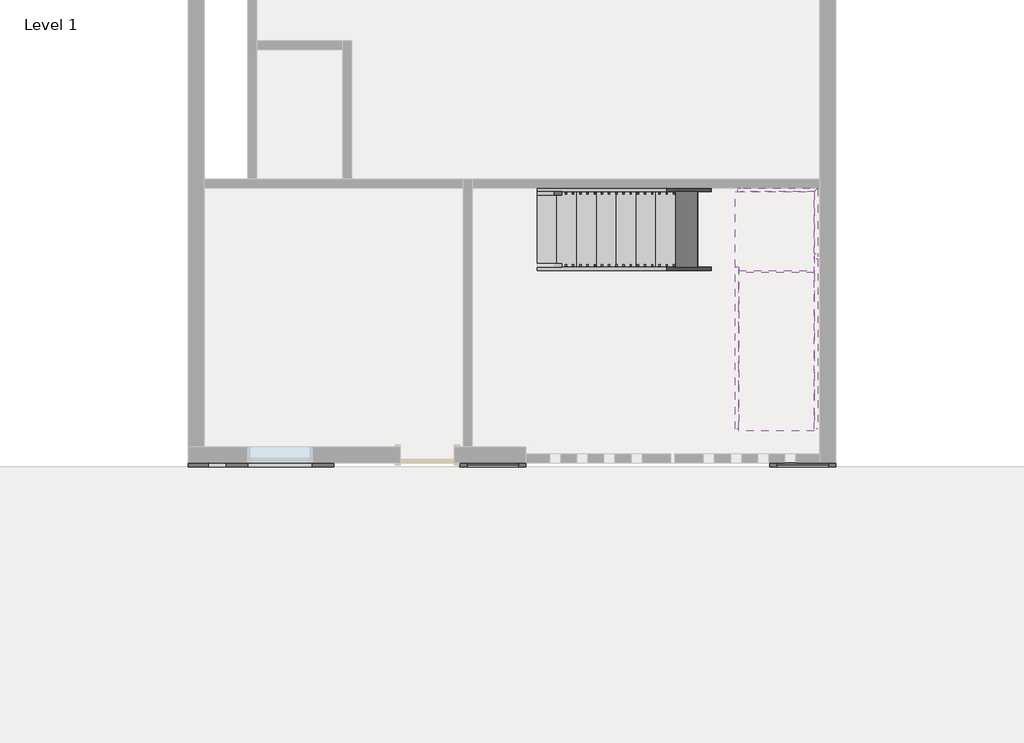
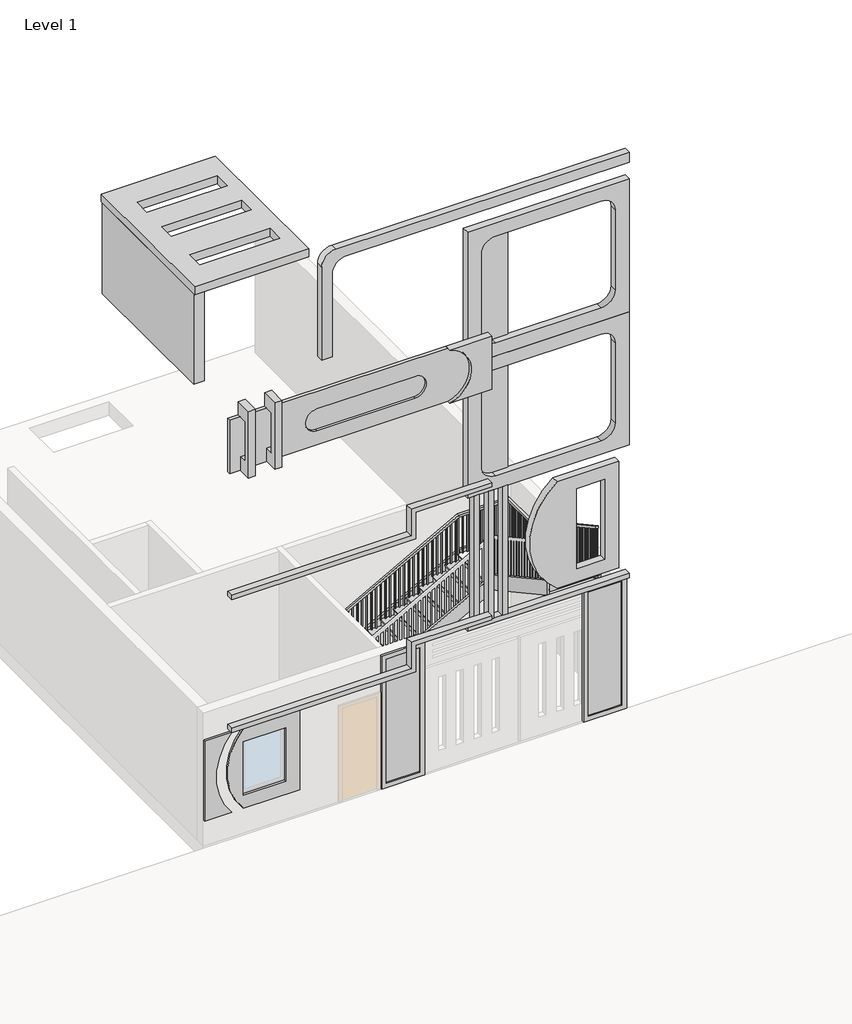
# One storey, part 2 of 2: 6 members, 2 stair flights, 1 proxy, 1 railing, 1 slab.
"""IFC4 building model written with IfcOpenShell, lengths in millimetres."""

from ifc_helpers import new_model, si_unit, frame, origin, place, context, project, spatial, polyline, outline, extrude, faceted_brep, transform, mapped, element, save
from components import generic_models_1_generic_models_1_57c6c2c0, non_monolithic_landing_2a78468c, stair_flight_cc90426c, stair_flight_f2f674f0

model = new_model("IFC4")

# Units and contexts
model_context = context("Model", 3, world=origin())
ifc_project = project(units=[si_unit("LENGTHUNIT", "METRE", prefix="MILLI")], contexts=[model_context])

# Site, building, storey
site = spatial("IfcSite", under=ifc_project)
building = spatial("IfcBuilding", under=site)
storey = spatial("IfcBuildingStorey", under=building, Name="Level 1", Elevation=0.0)

# Proxy
placement = place(None, origin())
generic_models_1_generic_models_1_shape = generic_models_1_generic_models_1_57c6c2c0(model_context)
element("IfcBuildingElementProxy", 1, Name="Generic Models 1 : Generic Models 1", ObjectType="Generic Models 1 : Generic Models 1", at=placement, inside=storey, context=model_context, shape_type="MappedRepresentation", body=[
    mapped(generic_models_1_generic_models_1_shape, transform((0.0, 0.0, 0.0), x_axis=(1.0, 0.0, 0.0), y_axis=(0.0, 1.0, 0.0), z_axis=(0.0, 0.0, 1.0))),
])

# Members
element("IfcMember", 2, ObjectType="Stringer - 2\" Width", at=placement, inside=storey, context=model_context, shape_type="SweptSolid", body=[
    extrude(outline(polyline([(206.7436667, -459.26646), (0.0, -459.26646), (0.0, -201.7743401), (1447.8, 2452.5256599), (1752.6, 2374.8034844), (206.7436667, -459.26646)])), frame((0.0, -782.3834702, 0.0), z_axis=(0.0, 1.0, 0.0), x_axis=(0.0, 0.0, 1.0)), (0.0, 0.0, 1.0), 50.8),
])
element("IfcMember", 3, ObjectType="Stringer - 2\" Width", at=placement, inside=storey, context=model_context, shape_type="SweptSolid", body=[
    extrude(outline(polyline([(206.7436667, -459.26646), (0.0, -459.26646), (0.0, -201.7743401), (1383.5497528, 2334.73354), (1730.7436667, 2334.73354), (206.7436667, -459.26646)])), frame((0.0, -1899.9834702, 0.0), z_axis=(0.0, 1.0, 0.0), x_axis=(0.0, 0.0, 1.0)), (0.0, 0.0, 1.0), 50.8),
])
element("IfcMember", 4, ObjectType="Stringer - 2\" Width", at=placement, inside=storey, context=model_context, shape_type="SweptSolid", body=[
    extrude(outline(polyline([(-1660.6534146, 1752.6), (-1738.3755901, 1447.8), (-4135.1834702, 2755.1497528), (-4135.1834702, 3102.3436667), (-1660.6534146, 1752.6)])), frame((3452.33354, 0.0, 0.0), z_axis=(1.0, 0.0, 0.0), x_axis=(0.0, 1.0, 0.0)), (0.0, 0.0, 1.0), 50.8),
])
element("IfcMember", 5, ObjectType="Stringer - 2\" Width", at=placement, inside=storey, context=model_context, shape_type="SweptSolid", body=[
    extrude(outline(polyline([(-1849.1834702, 1855.4345758), (-1849.1834702, 1508.2406619), (-4135.1834702, 2755.1497528), (-4135.1834702, 3102.3436667), (-1849.1834702, 1855.4345758)])), frame((2334.73354, 0.0, 0.0), z_axis=(1.0, 0.0, 0.0), x_axis=(0.0, 1.0, 0.0)), (0.0, 0.0, 1.0), 50.8),
])
element("IfcMember", 6, ObjectType="Stringer - 2\" Width", at=placement, inside=storey, context=model_context, shape_type="Brep", body=[
    faceted_brep([(3452.33354, -1660.6534146, 1752.6), (3503.13354, -1660.6534146, 1752.6), (3503.13354, -731.5834702, 1752.6), (3452.33354, -782.3834702, 1752.6), (3452.33354, -1738.3755901, 1447.8), (3452.33354, -782.3834702, 1447.8), (3503.13354, -1738.3755901, 1447.8), (3503.13354, -731.5834702, 1447.8)], [[[0, 1, 2, 3]], [[4, 0, 3, 5]], [[6, 4, 5, 7]], [[1, 6, 7, 2]], [[1, 0, 4, 6]], [[2, 7, 5, 3]]]),
])
element("IfcMember", 7, ObjectType="Stringer - 2\" Width", at=placement, inside=storey, context=model_context, shape_type="Brep", body=[
    faceted_brep([(3452.33354, -782.3834702, 1752.6), (3503.13354, -731.5834702, 1752.6), (2374.8034844, -731.5834702, 1752.6), (2374.8034844, -782.3834702, 1752.6), (3452.33354, -782.3834702, 1447.8), (2452.5256599, -782.3834702, 1447.8), (3503.13354, -731.5834702, 1447.8), (2452.5256599, -731.5834702, 1447.8)], [[[0, 1, 2, 3]], [[4, 0, 3, 5]], [[6, 4, 5, 7]], [[1, 6, 7, 2]], [[1, 0, 4, 6]], [[2, 7, 5, 3]]]),
])

# Railing
element("IfcRailing", 8, ObjectType="Handrail - Rectangular", at=placement, inside=storey, context=model_context, shape_type="SolidModel", body=[
    faceted_brep([(-459.26646, -782.3834702, 1066.8), (-459.26646, -782.3834702, 1008.9343477), (-459.26646, -833.1834702, 1008.9343477), (-459.26646, -833.1834702, 1066.8), (2334.73354, -782.3834702, 2590.8), (2347.687236, -782.3834702, 2540.0), (2347.687236, -833.1834702, 2540.0), (2334.73354, -833.1834702, 2590.8), (3452.33354, -782.3834702, 2590.8), (3452.33354, -782.3834702, 2540.0), (3401.53354, -833.1834702, 2540.0), (3401.53354, -833.1834702, 2590.8), (3452.33354, -1620.5834702, 2590.8), (3452.33354, -1633.5371661, 2540.0), (3401.53354, -1633.5371661, 2540.0), (3401.53354, -1620.5834702, 2590.8), (3452.33354, -1899.9834702, 2743.2), (3452.33354, -1924.3091585, 2698.6029049), (3401.53354, -1924.3091585, 2698.6029049), (3401.53354, -1899.9834702, 2743.2), (3452.33354, -4135.1834702, 3962.4), (3401.53354, -4135.1834702, 3962.4), (3401.53354, -4135.1834702, 3904.5343477), (3452.33354, -4135.1834702, 3904.5343477)], [[[0, 1, 2, 3]], [[1, 0, 4, 5]], [[2, 1, 5, 6]], [[3, 2, 6, 7]], [[0, 3, 7, 4]], [[5, 4, 8, 9]], [[6, 5, 9, 10]], [[7, 6, 10, 11]], [[4, 7, 11, 8]], [[9, 8, 12, 13]], [[10, 9, 13, 14]], [[11, 10, 14, 15]], [[8, 11, 15, 12]], [[13, 12, 16, 17]], [[14, 13, 17, 18]], [[15, 14, 18, 19]], [[12, 15, 19, 16]], [[20, 21, 22, 23]], [[17, 16, 20, 23]], [[18, 17, 23, 22]], [[19, 18, 22, 21]], [[16, 19, 21, 20]]]),
    extrude(outline(polyline([(-4024.0584702, 3843.9207113), (-4024.0584702, 2895.6), (-4043.1084702, 2895.6), (-4043.1084702, 3854.3116204), (-4024.0584702, 3843.9207113)])), frame((3417.40854, 0.0, 0.0), z_axis=(1.0, 0.0, 0.0), x_axis=(0.0, 1.0, 0.0)), (0.0, 0.0, 1.0), 19.05),
    extrude(outline(polyline([(-3922.4584702, 3788.5025295), (-3922.4584702, 2895.6), (-3941.5084702, 2895.6), (-3941.5084702, 3798.8934386), (-3922.4584702, 3788.5025295)])), frame((3417.40854, 0.0, 0.0), z_axis=(1.0, 0.0, 0.0), x_axis=(0.0, 1.0, 0.0)), (0.0, 0.0, 1.0), 19.05),
    extrude(outline(polyline([(-3820.8584702, 3733.0843477), (-3820.8584702, 2743.2), (-3839.9084702, 2743.2), (-3839.9084702, 3743.4752568), (-3820.8584702, 3733.0843477)])), frame((3417.40854, 0.0, 0.0), z_axis=(1.0, 0.0, 0.0), x_axis=(0.0, 1.0, 0.0)), (0.0, 0.0, 1.0), 19.05),
    extrude(outline(polyline([(-3719.2584702, 3677.6661659), (-3719.2584702, 2743.2), (-3738.3084702, 2743.2), (-3738.3084702, 3688.0570749), (-3719.2584702, 3677.6661659)])), frame((3417.40854, 0.0, 0.0), z_axis=(1.0, 0.0, 0.0), x_axis=(0.0, 1.0, 0.0)), (0.0, 0.0, 1.0), 19.05),
    extrude(outline(polyline([(-3617.6584702, 3622.247984), (-3617.6584702, 2743.2), (-3636.7084702, 2743.2), (-3636.7084702, 3632.6388931), (-3617.6584702, 3622.247984)])), frame((3417.40854, 0.0, 0.0), z_axis=(1.0, 0.0, 0.0), x_axis=(0.0, 1.0, 0.0)), (0.0, 0.0, 1.0), 19.05),
    extrude(outline(polyline([(-3516.0584702, 3566.8298022), (-3516.0584702, 2590.8), (-3535.1084702, 2590.8), (-3535.1084702, 3577.2207113), (-3516.0584702, 3566.8298022)])), frame((3417.40854, 0.0, 0.0), z_axis=(1.0, 0.0, 0.0), x_axis=(0.0, 1.0, 0.0)), (0.0, 0.0, 1.0), 19.05),
    extrude(outline(polyline([(-3414.4584702, 3511.4116204), (-3414.4584702, 2590.8), (-3433.5084702, 2590.8), (-3433.5084702, 3521.8025295), (-3414.4584702, 3511.4116204)])), frame((3417.40854, 0.0, 0.0), z_axis=(1.0, 0.0, 0.0), x_axis=(0.0, 1.0, 0.0)), (0.0, 0.0, 1.0), 19.05),
    extrude(outline(polyline([(-3312.8584702, 3455.9934386), (-3312.8584702, 2590.8), (-3331.9084702, 2590.8), (-3331.9084702, 3466.3843477), (-3312.8584702, 3455.9934386)])), frame((3417.40854, 0.0, 0.0), z_axis=(1.0, 0.0, 0.0), x_axis=(0.0, 1.0, 0.0)), (0.0, 0.0, 1.0), 19.05),
    extrude(outline(polyline([(-3211.2584702, 3400.5752568), (-3211.2584702, 2438.4), (-3230.3084702, 2438.4), (-3230.3084702, 3410.9661659), (-3211.2584702, 3400.5752568)])), frame((3417.40854, 0.0, 0.0), z_axis=(1.0, 0.0, 0.0), x_axis=(0.0, 1.0, 0.0)), (0.0, 0.0, 1.0), 19.05),
    extrude(outline(polyline([(-3109.6584702, 3345.1570749), (-3109.6584702, 2438.4), (-3128.7084702, 2438.4), (-3128.7084702, 3355.547984), (-3109.6584702, 3345.1570749)])), frame((3417.40854, 0.0, 0.0), z_axis=(1.0, 0.0, 0.0), x_axis=(0.0, 1.0, 0.0)), (0.0, 0.0, 1.0), 19.05),
    extrude(outline(polyline([(-3008.0584702, 3289.7388931), (-3008.0584702, 2438.4), (-3027.1084702, 2438.4), (-3027.1084702, 3300.1298022), (-3008.0584702, 3289.7388931)])), frame((3417.40854, 0.0, 0.0), z_axis=(1.0, 0.0, 0.0), x_axis=(0.0, 1.0, 0.0)), (0.0, 0.0, 1.0), 19.05),
    extrude(outline(polyline([(-2906.4584702, 3234.3207113), (-2906.4584702, 2286.0), (-2925.5084702, 2286.0), (-2925.5084702, 3244.7116204), (-2906.4584702, 3234.3207113)])), frame((3417.40854, 0.0, 0.0), z_axis=(1.0, 0.0, 0.0), x_axis=(0.0, 1.0, 0.0)), (0.0, 0.0, 1.0), 19.05),
    extrude(outline(polyline([(-2804.8584702, 3178.9025295), (-2804.8584702, 2286.0), (-2823.9084702, 2286.0), (-2823.9084702, 3189.2934386), (-2804.8584702, 3178.9025295)])), frame((3417.40854, 0.0, 0.0), z_axis=(1.0, 0.0, 0.0), x_axis=(0.0, 1.0, 0.0)), (0.0, 0.0, 1.0), 19.05),
    extrude(outline(polyline([(-2703.2584702, 3123.4843477), (-2703.2584702, 2133.6), (-2722.3084702, 2133.6), (-2722.3084702, 3133.8752568), (-2703.2584702, 3123.4843477)])), frame((3417.40854, 0.0, 0.0), z_axis=(1.0, 0.0, 0.0), x_axis=(0.0, 1.0, 0.0)), (0.0, 0.0, 1.0), 19.05),
    extrude(outline(polyline([(-2601.6584702, 3068.0661659), (-2601.6584702, 2133.6), (-2620.7084702, 2133.6), (-2620.7084702, 3078.4570749), (-2601.6584702, 3068.0661659)])), frame((3417.40854, 0.0, 0.0), z_axis=(1.0, 0.0, 0.0), x_axis=(0.0, 1.0, 0.0)), (0.0, 0.0, 1.0), 19.05),
    extrude(outline(polyline([(-2500.0584702, 3012.647984), (-2500.0584702, 2133.6), (-2519.1084702, 2133.6), (-2519.1084702, 3023.0388931), (-2500.0584702, 3012.647984)])), frame((3417.40854, 0.0, 0.0), z_axis=(1.0, 0.0, 0.0), x_axis=(0.0, 1.0, 0.0)), (0.0, 0.0, 1.0), 19.05),
    extrude(outline(polyline([(-2398.4584702, 2957.2298022), (-2398.4584702, 1981.2), (-2417.5084702, 1981.2), (-2417.5084702, 2967.6207113), (-2398.4584702, 2957.2298022)])), frame((3417.40854, 0.0, 0.0), z_axis=(1.0, 0.0, 0.0), x_axis=(0.0, 1.0, 0.0)), (0.0, 0.0, 1.0), 19.05),
    extrude(outline(polyline([(-2296.8584702, 2901.8116204), (-2296.8584702, 1981.2), (-2315.9084702, 1981.2), (-2315.9084702, 2912.2025295), (-2296.8584702, 2901.8116204)])), frame((3417.40854, 0.0, 0.0), z_axis=(1.0, 0.0, 0.0), x_axis=(0.0, 1.0, 0.0)), (0.0, 0.0, 1.0), 19.05),
    extrude(outline(polyline([(-2195.2584702, 2846.3934386), (-2195.2584702, 1981.2), (-2214.3084702, 1981.2), (-2214.3084702, 2856.7843477), (-2195.2584702, 2846.3934386)])), frame((3417.40854, 0.0, 0.0), z_axis=(1.0, 0.0, 0.0), x_axis=(0.0, 1.0, 0.0)), (0.0, 0.0, 1.0), 19.05),
    extrude(outline(polyline([(-2093.6584702, 2790.9752568), (-2093.6584702, 1828.8), (-2112.7084702, 1828.8), (-2112.7084702, 2801.3661659), (-2093.6584702, 2790.9752568)])), frame((3417.40854, 0.0, 0.0), z_axis=(1.0, 0.0, 0.0), x_axis=(0.0, 1.0, 0.0)), (0.0, 0.0, 1.0), 19.05),
    extrude(outline(polyline([(-1992.0584702, 2735.5570749), (-1992.0584702, 1828.8), (-2011.1084702, 1828.8), (-2011.1084702, 2745.947984), (-1992.0584702, 2735.5570749)])), frame((3417.40854, 0.0, 0.0), z_axis=(1.0, 0.0, 0.0), x_axis=(0.0, 1.0, 0.0)), (0.0, 0.0, 1.0), 19.05),
    extrude(outline(polyline([(-1814.2584702, 2638.5752568), (-1814.2584702, 1676.4), (-1833.3084702, 1676.4), (-1833.3084702, 2648.9661659), (-1814.2584702, 2638.5752568)])), frame((3417.40854, 0.0, 0.0), z_axis=(1.0, 0.0, 0.0), x_axis=(0.0, 1.0, 0.0)), (0.0, 0.0, 1.0), 19.05),
    extrude(outline(polyline([(-1712.6584702, 2583.1570749), (-1712.6584702, 1676.4), (-1731.7084702, 1676.4), (-1731.7084702, 2593.547984), (-1712.6584702, 2583.1570749)])), frame((3417.40854, 0.0, 0.0), z_axis=(1.0, 0.0, 0.0), x_axis=(0.0, 1.0, 0.0)), (0.0, 0.0, 1.0), 19.05),
    extrude(outline(polyline([(3436.45854, -1611.0584702), (3436.45854, -1630.1084702), (3417.40854, -1630.1084702), (3417.40854, -1611.0584702), (3436.45854, -1611.0584702)])), frame((0.0, 0.0, 1676.4), z_axis=(0.0, 0.0, 1.0), x_axis=(1.0, 0.0, 0.0)), (0.0, 0.0, 1.0), 863.6),
    extrude(outline(polyline([(3436.45854, -1509.4584702), (3436.45854, -1528.5084702), (3417.40854, -1528.5084702), (3417.40854, -1509.4584702), (3436.45854, -1509.4584702)])), frame((0.0, 0.0, 1676.4), z_axis=(0.0, 0.0, 1.0), x_axis=(1.0, 0.0, 0.0)), (0.0, 0.0, 1.0), 863.6),
    extrude(outline(polyline([(3436.45854, -1407.8584702), (3436.45854, -1426.9084702), (3417.40854, -1426.9084702), (3417.40854, -1407.8584702), (3436.45854, -1407.8584702)])), frame((0.0, 0.0, 1676.4), z_axis=(0.0, 0.0, 1.0), x_axis=(1.0, 0.0, 0.0)), (0.0, 0.0, 1.0), 863.6),
    extrude(outline(polyline([(3436.45854, -1306.2584702), (3436.45854, -1325.3084702), (3417.40854, -1325.3084702), (3417.40854, -1306.2584702), (3436.45854, -1306.2584702)])), frame((0.0, 0.0, 1676.4), z_axis=(0.0, 0.0, 1.0), x_axis=(1.0, 0.0, 0.0)), (0.0, 0.0, 1.0), 863.6),
    extrude(outline(polyline([(3436.45854, -1204.6584702), (3436.45854, -1223.7084702), (3417.40854, -1223.7084702), (3417.40854, -1204.6584702), (3436.45854, -1204.6584702)])), frame((0.0, 0.0, 1676.4), z_axis=(0.0, 0.0, 1.0), x_axis=(1.0, 0.0, 0.0)), (0.0, 0.0, 1.0), 863.6),
    extrude(outline(polyline([(3436.45854, -1103.0584702), (3436.45854, -1122.1084702), (3417.40854, -1122.1084702), (3417.40854, -1103.0584702), (3436.45854, -1103.0584702)])), frame((0.0, 0.0, 1676.4), z_axis=(0.0, 0.0, 1.0), x_axis=(1.0, 0.0, 0.0)), (0.0, 0.0, 1.0), 863.6),
    extrude(outline(polyline([(3436.45854, -1001.4584702), (3436.45854, -1020.5084702), (3417.40854, -1020.5084702), (3417.40854, -1001.4584702), (3436.45854, -1001.4584702)])), frame((0.0, 0.0, 1676.4), z_axis=(0.0, 0.0, 1.0), x_axis=(1.0, 0.0, 0.0)), (0.0, 0.0, 1.0), 863.6),
    extrude(outline(polyline([(3436.45854, -899.8584702), (3436.45854, -918.9084702), (3417.40854, -918.9084702), (3417.40854, -899.8584702), (3436.45854, -899.8584702)])), frame((0.0, 0.0, 1676.4), z_axis=(0.0, 0.0, 1.0), x_axis=(1.0, 0.0, 0.0)), (0.0, 0.0, 1.0), 863.6),
    extrude(outline(polyline([(3341.20854, -798.2584702), (3360.25854, -798.2584702), (3360.25854, -817.3084702), (3341.20854, -817.3084702), (3341.20854, -798.2584702)])), frame((0.0, 0.0, 1676.4), z_axis=(0.0, 0.0, 1.0), x_axis=(1.0, 0.0, 0.0)), (0.0, 0.0, 1.0), 863.6),
    extrude(outline(polyline([(3239.60854, -798.2584702), (3258.65854, -798.2584702), (3258.65854, -817.3084702), (3239.60854, -817.3084702), (3239.60854, -798.2584702)])), frame((0.0, 0.0, 1676.4), z_axis=(0.0, 0.0, 1.0), x_axis=(1.0, 0.0, 0.0)), (0.0, 0.0, 1.0), 863.6),
    extrude(outline(polyline([(3138.00854, -798.2584702), (3157.05854, -798.2584702), (3157.05854, -817.3084702), (3138.00854, -817.3084702), (3138.00854, -798.2584702)])), frame((0.0, 0.0, 1676.4), z_axis=(0.0, 0.0, 1.0), x_axis=(1.0, 0.0, 0.0)), (0.0, 0.0, 1.0), 863.6),
    extrude(outline(polyline([(3036.40854, -798.2584702), (3055.45854, -798.2584702), (3055.45854, -817.3084702), (3036.40854, -817.3084702), (3036.40854, -798.2584702)])), frame((0.0, 0.0, 1676.4), z_axis=(0.0, 0.0, 1.0), x_axis=(1.0, 0.0, 0.0)), (0.0, 0.0, 1.0), 863.6),
    extrude(outline(polyline([(2934.80854, -798.2584702), (2953.85854, -798.2584702), (2953.85854, -817.3084702), (2934.80854, -817.3084702), (2934.80854, -798.2584702)])), frame((0.0, 0.0, 1676.4), z_axis=(0.0, 0.0, 1.0), x_axis=(1.0, 0.0, 0.0)), (0.0, 0.0, 1.0), 863.6),
    extrude(outline(polyline([(2833.20854, -798.2584702), (2852.25854, -798.2584702), (2852.25854, -817.3084702), (2833.20854, -817.3084702), (2833.20854, -798.2584702)])), frame((0.0, 0.0, 1676.4), z_axis=(0.0, 0.0, 1.0), x_axis=(1.0, 0.0, 0.0)), (0.0, 0.0, 1.0), 863.6),
    extrude(outline(polyline([(2731.60854, -798.2584702), (2750.65854, -798.2584702), (2750.65854, -817.3084702), (2731.60854, -817.3084702), (2731.60854, -798.2584702)])), frame((0.0, 0.0, 1676.4), z_axis=(0.0, 0.0, 1.0), x_axis=(1.0, 0.0, 0.0)), (0.0, 0.0, 1.0), 863.6),
    extrude(outline(polyline([(2630.00854, -798.2584702), (2649.05854, -798.2584702), (2649.05854, -817.3084702), (2630.00854, -817.3084702), (2630.00854, -798.2584702)])), frame((0.0, 0.0, 1676.4), z_axis=(0.0, 0.0, 1.0), x_axis=(1.0, 0.0, 0.0)), (0.0, 0.0, 1.0), 863.6),
    extrude(outline(polyline([(2528.40854, -798.2584702), (2547.45854, -798.2584702), (2547.45854, -817.3084702), (2528.40854, -817.3084702), (2528.40854, -798.2584702)])), frame((0.0, 0.0, 1676.4), z_axis=(0.0, 0.0, 1.0), x_axis=(1.0, 0.0, 0.0)), (0.0, 0.0, 1.0), 863.6),
    extrude(outline(polyline([(2426.80854, -798.2584702), (2445.85854, -798.2584702), (2445.85854, -817.3084702), (2426.80854, -817.3084702), (2426.80854, -798.2584702)])), frame((0.0, 0.0, 1676.4), z_axis=(0.0, 0.0, 1.0), x_axis=(1.0, 0.0, 0.0)), (0.0, 0.0, 1.0), 863.6),
    extrude(outline(polyline([(2500.0298022, 2274.40854), (1524.0, 2274.40854), (1524.0, 2293.45854), (2510.4207113, 2293.45854), (2500.0298022, 2274.40854)])), frame((0.0, -817.3084702, 0.0), z_axis=(0.0, 1.0, 0.0), x_axis=(0.0, 0.0, 1.0)), (0.0, 0.0, 1.0), 19.05),
    extrude(outline(polyline([(2444.6116204, 2172.80854), (1524.0, 2172.80854), (1524.0, 2191.85854), (2455.0025295, 2191.85854), (2444.6116204, 2172.80854)])), frame((0.0, -817.3084702, 0.0), z_axis=(0.0, 1.0, 0.0), x_axis=(0.0, 0.0, 1.0)), (0.0, 0.0, 1.0), 19.05),
    extrude(outline(polyline([(2389.1934386, 2071.20854), (1524.0, 2071.20854), (1524.0, 2090.25854), (2399.5843477, 2090.25854), (2389.1934386, 2071.20854)])), frame((0.0, -817.3084702, 0.0), z_axis=(0.0, 1.0, 0.0), x_axis=(0.0, 0.0, 1.0)), (0.0, 0.0, 1.0), 19.05),
    extrude(outline(polyline([(2333.7752568, 1969.60854), (1371.6, 1969.60854), (1371.6, 1988.65854), (2344.1661659, 1988.65854), (2333.7752568, 1969.60854)])), frame((0.0, -817.3084702, 0.0), z_axis=(0.0, 1.0, 0.0), x_axis=(0.0, 0.0, 1.0)), (0.0, 0.0, 1.0), 19.05),
    extrude(outline(polyline([(2278.3570749, 1868.00854), (1371.6, 1868.00854), (1371.6, 1887.05854), (2288.747984, 1887.05854), (2278.3570749, 1868.00854)])), frame((0.0, -817.3084702, 0.0), z_axis=(0.0, 1.0, 0.0), x_axis=(0.0, 0.0, 1.0)), (0.0, 0.0, 1.0), 19.05),
    extrude(outline(polyline([(2222.9388931, 1766.40854), (1371.6, 1766.40854), (1371.6, 1785.45854), (2233.3298022, 1785.45854), (2222.9388931, 1766.40854)])), frame((0.0, -817.3084702, 0.0), z_axis=(0.0, 1.0, 0.0), x_axis=(0.0, 0.0, 1.0)), (0.0, 0.0, 1.0), 19.05),
    extrude(outline(polyline([(2167.5207113, 1664.80854), (1219.2, 1664.80854), (1219.2, 1683.85854), (2177.9116204, 1683.85854), (2167.5207113, 1664.80854)])), frame((0.0, -817.3084702, 0.0), z_axis=(0.0, 1.0, 0.0), x_axis=(0.0, 0.0, 1.0)), (0.0, 0.0, 1.0), 19.05),
    extrude(outline(polyline([(2112.1025295, 1563.20854), (1219.2, 1563.20854), (1219.2, 1582.25854), (2122.4934386, 1582.25854), (2112.1025295, 1563.20854)])), frame((0.0, -817.3084702, 0.0), z_axis=(0.0, 1.0, 0.0), x_axis=(0.0, 0.0, 1.0)), (0.0, 0.0, 1.0), 19.05),
    extrude(outline(polyline([(2056.6843477, 1461.60854), (1066.8, 1461.60854), (1066.8, 1480.65854), (2067.0752568, 1480.65854), (2056.6843477, 1461.60854)])), frame((0.0, -817.3084702, 0.0), z_axis=(0.0, 1.0, 0.0), x_axis=(0.0, 0.0, 1.0)), (0.0, 0.0, 1.0), 19.05),
    extrude(outline(polyline([(2001.2661659, 1360.00854), (1066.8, 1360.00854), (1066.8, 1379.05854), (2011.6570749, 1379.05854), (2001.2661659, 1360.00854)])), frame((0.0, -817.3084702, 0.0), z_axis=(0.0, 1.0, 0.0), x_axis=(0.0, 0.0, 1.0)), (0.0, 0.0, 1.0), 19.05),
    extrude(outline(polyline([(1945.847984, 1258.40854), (1066.8, 1258.40854), (1066.8, 1277.45854), (1956.2388931, 1277.45854), (1945.847984, 1258.40854)])), frame((0.0, -817.3084702, 0.0), z_axis=(0.0, 1.0, 0.0), x_axis=(0.0, 0.0, 1.0)), (0.0, 0.0, 1.0), 19.05),
    extrude(outline(polyline([(1890.4298022, 1156.80854), (914.4, 1156.80854), (914.4, 1175.85854), (1900.8207113, 1175.85854), (1890.4298022, 1156.80854)])), frame((0.0, -817.3084702, 0.0), z_axis=(0.0, 1.0, 0.0), x_axis=(0.0, 0.0, 1.0)), (0.0, 0.0, 1.0), 19.05),
    extrude(outline(polyline([(1835.0116204, 1055.20854), (914.4, 1055.20854), (914.4, 1074.25854), (1845.4025295, 1074.25854), (1835.0116204, 1055.20854)])), frame((0.0, -817.3084702, 0.0), z_axis=(0.0, 1.0, 0.0), x_axis=(0.0, 0.0, 1.0)), (0.0, 0.0, 1.0), 19.05),
    extrude(outline(polyline([(1779.5934386, 953.60854), (914.4, 953.60854), (914.4, 972.65854), (1789.9843477, 972.65854), (1779.5934386, 953.60854)])), frame((0.0, -817.3084702, 0.0), z_axis=(0.0, 1.0, 0.0), x_axis=(0.0, 0.0, 1.0)), (0.0, 0.0, 1.0), 19.05),
    extrude(outline(polyline([(1724.1752568, 852.00854), (762.0, 852.00854), (762.0, 871.05854), (1734.5661659, 871.05854), (1724.1752568, 852.00854)])), frame((0.0, -817.3084702, 0.0), z_axis=(0.0, 1.0, 0.0), x_axis=(0.0, 0.0, 1.0)), (0.0, 0.0, 1.0), 19.05),
    extrude(outline(polyline([(1668.7570749, 750.40854), (762.0, 750.40854), (762.0, 769.45854), (1679.147984, 769.45854), (1668.7570749, 750.40854)])), frame((0.0, -817.3084702, 0.0), z_axis=(0.0, 1.0, 0.0), x_axis=(0.0, 0.0, 1.0)), (0.0, 0.0, 1.0), 19.05),
    extrude(outline(polyline([(1613.3388931, 648.80854), (762.0, 648.80854), (762.0, 667.85854), (1623.7298022, 667.85854), (1613.3388931, 648.80854)])), frame((0.0, -817.3084702, 0.0), z_axis=(0.0, 1.0, 0.0), x_axis=(0.0, 0.0, 1.0)), (0.0, 0.0, 1.0), 19.05),
    extrude(outline(polyline([(1557.9207113, 547.20854), (609.6, 547.20854), (609.6, 566.25854), (1568.3116204, 566.25854), (1557.9207113, 547.20854)])), frame((0.0, -817.3084702, 0.0), z_axis=(0.0, 1.0, 0.0), x_axis=(0.0, 0.0, 1.0)), (0.0, 0.0, 1.0), 19.05),
    extrude(outline(polyline([(1502.5025295, 445.60854), (609.6, 445.60854), (609.6, 464.65854), (1512.8934386, 464.65854), (1502.5025295, 445.60854)])), frame((0.0, -817.3084702, 0.0), z_axis=(0.0, 1.0, 0.0), x_axis=(0.0, 0.0, 1.0)), (0.0, 0.0, 1.0), 19.05),
    extrude(outline(polyline([(1447.0843477, 344.00854), (457.2, 344.00854), (457.2, 363.05854), (1457.4752568, 363.05854), (1447.0843477, 344.00854)])), frame((0.0, -817.3084702, 0.0), z_axis=(0.0, 1.0, 0.0), x_axis=(0.0, 0.0, 1.0)), (0.0, 0.0, 1.0), 19.05),
    extrude(outline(polyline([(1391.6661659, 242.40854), (457.2, 242.40854), (457.2, 261.45854), (1402.0570749, 261.45854), (1391.6661659, 242.40854)])), frame((0.0, -817.3084702, 0.0), z_axis=(0.0, 1.0, 0.0), x_axis=(0.0, 0.0, 1.0)), (0.0, 0.0, 1.0), 19.05),
    extrude(outline(polyline([(1336.247984, 140.80854), (457.2, 140.80854), (457.2, 159.85854), (1346.6388931, 159.85854), (1336.247984, 140.80854)])), frame((0.0, -817.3084702, 0.0), z_axis=(0.0, 1.0, 0.0), x_axis=(0.0, 0.0, 1.0)), (0.0, 0.0, 1.0), 19.05),
    extrude(outline(polyline([(1280.8298022, 39.20854), (304.8, 39.20854), (304.8, 58.25854), (1291.2207113, 58.25854), (1280.8298022, 39.20854)])), frame((0.0, -817.3084702, 0.0), z_axis=(0.0, 1.0, 0.0), x_axis=(0.0, 0.0, 1.0)), (0.0, 0.0, 1.0), 19.05),
    extrude(outline(polyline([(1225.4116204, -62.39146), (304.8, -62.39146), (304.8, -43.34146), (1235.8025295, -43.34146), (1225.4116204, -62.39146)])), frame((0.0, -817.3084702, 0.0), z_axis=(0.0, 1.0, 0.0), x_axis=(0.0, 0.0, 1.0)), (0.0, 0.0, 1.0), 19.05),
    extrude(outline(polyline([(1169.9934386, -163.99146), (304.8, -163.99146), (304.8, -144.94146), (1180.3843477, -144.94146), (1169.9934386, -163.99146)])), frame((0.0, -817.3084702, 0.0), z_axis=(0.0, 1.0, 0.0), x_axis=(0.0, 0.0, 1.0)), (0.0, 0.0, 1.0), 19.05),
    extrude(outline(polyline([(1114.5752568, -265.59146), (152.4, -265.59146), (152.4, -246.54146), (1124.9661659, -246.54146), (1114.5752568, -265.59146)])), frame((0.0, -817.3084702, 0.0), z_axis=(0.0, 1.0, 0.0), x_axis=(0.0, 0.0, 1.0)), (0.0, 0.0, 1.0), 19.05),
    extrude(outline(polyline([(1059.1570749, -367.19146), (152.4, -367.19146), (152.4, -348.14146), (1069.547984, -348.14146), (1059.1570749, -367.19146)])), frame((0.0, -817.3084702, 0.0), z_axis=(0.0, 1.0, 0.0), x_axis=(0.0, 0.0, 1.0)), (0.0, 0.0, 1.0), 19.05),
    extrude(outline(polyline([(-1890.4584702, 2680.1388931), (-1890.4584702, 1676.4), (-1909.5084702, 1676.4), (-1909.5084702, 2690.5298022), (-1890.4584702, 2680.1388931)])), frame((3417.40854, 0.0, 0.0), z_axis=(1.0, 0.0, 0.0), x_axis=(0.0, 1.0, 0.0)), (0.0, 0.0, 1.0), 19.05),
    extrude(outline(polyline([(3417.40854, -798.2584702), (3436.45854, -798.2584702), (3436.45854, -817.3084702), (3417.40854, -817.3084702), (3417.40854, -798.2584702)])), frame((0.0, 0.0, 1676.4), z_axis=(0.0, 0.0, 1.0), x_axis=(1.0, 0.0, 0.0)), (0.0, 0.0, 1.0), 863.6),
    extrude(outline(polyline([(2527.7388931, 2325.20854), (1676.4, 2325.20854), (1676.4, 2344.25854), (2538.1298022, 2344.25854), (2527.7388931, 2325.20854)])), frame((0.0, -817.3084702, 0.0), z_axis=(0.0, 1.0, 0.0), x_axis=(0.0, 0.0, 1.0)), (0.0, 0.0, 1.0), 19.05),
    extrude(outline(polyline([(-4116.1334702, 3894.1434386), (-4116.1334702, 2895.6), (-4135.1834702, 2895.6), (-4135.1834702, 3904.5343477), (-4116.1334702, 3894.1434386)])), frame((3417.40854, 0.0, 0.0), z_axis=(1.0, 0.0, 0.0), x_axis=(0.0, 1.0, 0.0)), (0.0, 0.0, 1.0), 19.05),
    extrude(outline(polyline([(1008.9343477, -459.26646), (152.4, -459.26646), (152.4, -440.21646), (1019.3252568, -440.21646), (1008.9343477, -459.26646)])), frame((0.0, -817.3084702, 0.0), z_axis=(0.0, 1.0, 0.0), x_axis=(0.0, 0.0, 1.0)), (0.0, 0.0, 1.0), 19.05),
])

# Slab
non_monolithic_landing_shape = non_monolithic_landing_2a78468c(model_context)
element("IfcSlab", 9, ObjectType="Non-Monolithic Landing", at=placement, inside=storey, context=model_context, shape_type="MappedRepresentation", body=[
    mapped(non_monolithic_landing_shape, transform((0.0, 0.0, 0.0), x_axis=(1.0, 0.0, 0.0), y_axis=(0.0, 1.0, 0.0), z_axis=(0.0, 0.0, 1.0))),
])

# Stair flights
stair_flight_shape = stair_flight_cc90426c(model_context)
element("IfcStairFlight", 10, ObjectType="2\" Tread 1\" Nosing 1/4\" Riser", at=placement, inside=storey, context=model_context, shape_type="MappedRepresentation", body=[
    mapped(stair_flight_shape, transform((0.0, 0.0, 0.0), x_axis=(1.0, 0.0, 0.0), y_axis=(0.0, 1.0, 0.0), z_axis=(0.0, 0.0, 1.0))),
])
stair_flight_2_shape = stair_flight_f2f674f0(model_context)
element("IfcStairFlight", 11, ObjectType="2\" Tread 1\" Nosing 1/4\" Riser", at=placement, inside=storey, context=model_context, shape_type="MappedRepresentation", body=[
    mapped(stair_flight_2_shape, transform((0.0, 0.0, 0.0), x_axis=(1.0, 0.0, 0.0), y_axis=(0.0, 1.0, 0.0), z_axis=(0.0, 0.0, 1.0))),
])

save(model, "model.ifc")

# Revit data of these elements
# Type "Handrail - Rectangular"
#   Assembly Code = "C2010400"
#   built-in parameter 1008612 = 0.0416667 (stored number, unit not read)
#   built-in parameter 1008611 = 0.0416667 (stored number, unit not read)
#   built-in parameter 1008609 = 0.333333 (stored number, unit not read)
#   built-in parameter 1008604 = 0.166667 (stored number, unit not read)
#   built-in parameter 1008603 = 0.166667 (stored number, unit not read)
#   Railing Height = 3' - 0"
#   built-in parameter 1008630 = 2
#   built-in parameter 1008610 = 2
#   built-in parameter 1008618 = Baluster - Square : 3/4"
# Element 1 (IfcBuildingElementProxy, "Generic Models 1 : Generic Models 1")
#   Phase Created = New Construction
#   Materials on its faces: "03 white", "02 colour", "04 tiles", "01 colour"
# Elements 2, 3, 4, 5, 6, 7 (IfcMember, "Stringer - 2\" Width")
#   Phase Created = New Construction
# Element 8 (IfcRailing, "Handrail - Rectangular")
#   Phase Created = New Construction
# Element 9 (IfcSlab, "Non-Monolithic Landing")
#   Phase Created = New Construction
# Elements 10, 11 (IfcStairFlight, "2\" Tread 1\" Nosing 1/4\" Riser")
#   Phase Created = New Construction
# Materials
#   "03 white": class "Generic", colour RGB 120 120 120, transparency 0, Cost = 0
#   "02 colour": class "Generic", colour RGB 120 120 120, transparency 0, Cost = 0
#   "04 tiles": class "Generic", colour RGB 120 120 120, transparency 0, Cost = 0
#   "01 colour": class "Generic", colour RGB 120 120 120, transparency 0, Cost = 0
